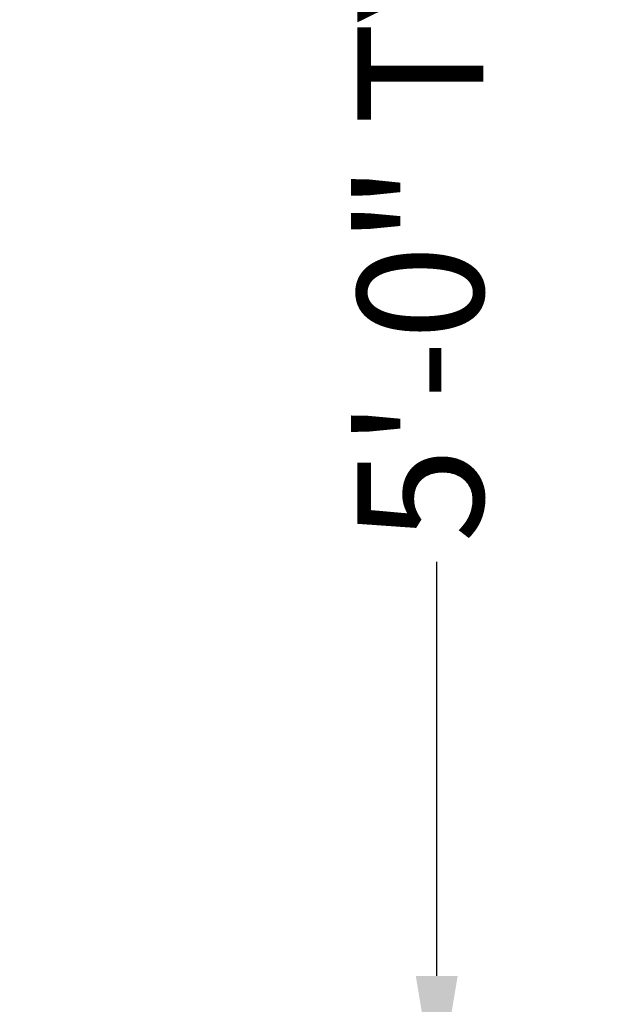
# Model space of a CAD drawing. Units: inches. Extents: x -638 to 186, y -762 to 59.
# Tile 27 of 31: x -46 to -27, y -108 to -77. Entities that reach past the tile are written whole.
import ezdxf

# ---------------------------------------------------------------- set-up
doc = ezdxf.new("R2010")
doc.units = ezdxf.units.IN
doc.layers.add('A-ANNO-DIMS', color=2, linetype='Continuous', lineweight=18)
doc.styles.get("Standard").update_dxf_attribs({"font": 'arial.ttf'})
doc.dimstyles.new('ISO-25', dxfattribs={"dimtxt": 4, "dimasz": 4, "dimexe": 1.25, "dimexo": 0.625, "dimtad": 0, "dimlunit": 4, "dimtxsty": 'Standard', "dimcen": 2.5, "dimclrt": 256, "dimadec": 0, "dimazin": 0, "dimtfac": 1, "dimtmove": 0, "dimatfit": 3, "dimfxl": 1, "dimfxlon": 1, "dimarcsym": 0})

# ---------------------------------------------------------------- blocks, each defined once
blk = doc.blocks.new('*D27')
at = {"layer": 'A-ANNO-DIMS', "color": 0, "lineweight": -2, "transparency": 16777216}
for p, q in [((-123.625, -121.818), (-123.625, -124.068)), ((-44.925, -121.818), (-44.925, -124.068)), ((-119.625, -122.818), (-114.394, -122.818)), ((-48.925, -122.818), (-54.156, -122.818))]:
    blk.add_line(p, q, dxfattribs=at)
at = {"layer": 'A-ANNO-DIMS', "color": 0, "lineweight": 30, "transparency": 16777216}
for points in [[(-119.625, -122.151), (-119.625, -123.485), (-123.625, -122.818)], [(-48.925, -122.151), (-48.925, -123.485), (-44.925, -122.818)]]:
    blk.add_solid(points, dxfattribs=at)
at = {"layer": 'Defpoints', "color": 0, "lineweight": 30, "transparency": 16777216}
for p in [(-123.625, -111.013), (-44.925, -111.013), (-44.925, -122.818)]:
    blk.add_point(p, dxfattribs=at)
at = {"layer": 'A-ANNO-DIMS', "transparency": 16777216, "insert": (-84.275, -122.818), "char_height": 4, "attachment_point": 5}
blk.add_mtext('BED SET 6\'-6 1/2" TYP.', dxfattribs=at)
blk = doc.blocks.new('*D28')
at = {"layer": 'A-ANNO-DIMS', "color": 0, "lineweight": -2, "transparency": 16777216}
for p, q in [((-34.121, -51.062), (-31.871, -51.062)), ((-33.121, -55.062), (-33.121, -68.221)), ((-33.121, -107.013), (-33.121, -93.853)), ((-34.121, -111.013), (-31.871, -111.013))]:
    blk.add_line(p, q, dxfattribs=at)
at = {"layer": 'A-ANNO-DIMS', "color": 0, "lineweight": 30, "transparency": 16777216}
for points in [[(-33.787, -55.062), (-32.454, -55.062), (-33.121, -51.062)], [(-33.787, -107.013), (-32.454, -107.013), (-33.121, -111.013)]]:
    blk.add_solid(points, dxfattribs=at)
at = {"layer": 'Defpoints', "color": 0, "lineweight": 30, "transparency": 16777216}
for p in [(-44.925, -51.062), (-33.121, -51.062), (-44.925, -111.013)]:
    blk.add_point(p, dxfattribs=at)
at = {"layer": 'A-ANNO-DIMS', "transparency": 16777216, "insert": (-33.121, -81.037), "char_height": 4, "attachment_point": 5, "rotation": 90}
blk.add_mtext('5\'-0" TYP.', dxfattribs=at)

msp = doc.modelspace()

# ---------------------------------------------------------------- dimensions: what is measured, and where the dimension line sits
at = {"layer": 'A-ANNO-DIMS'}
dim = msp.add_linear_dim(base=(-33.121, -51.062), p1=(-44.925, -111.013), p2=(-44.925, -51.062), angle=90, text='<> TYP.', dimstyle='ISO-25', override={"dimdec": 1, "dimlfac": 1, "dimrnd": 0, "dimzin": 1, "dimdsep": 46, "dimlunit": 4, "dimfrac": 2}, dxfattribs=at)
dim.commit()
dim.dimension.update_dxf_attribs({"geometry": '*D28', "text_midpoint": (-33.121, -81.037)})
dim = msp.add_linear_dim(base=(-44.925, -122.818), p1=(-123.625, -111.013), p2=(-44.925, -111.013), text='BED SET <> TYP.', dimstyle='ISO-25', override={"dimdec": 1, "dimlfac": 1, "dimrnd": 0, "dimzin": 1, "dimdsep": 46, "dimlunit": 4, "dimfrac": 2}, dxfattribs=at)
dim.commit()
dim.dimension.update_dxf_attribs({"geometry": '*D27', "text_midpoint": (-84.275, -122.818)})

doc.saveas('drawing.dxf')
